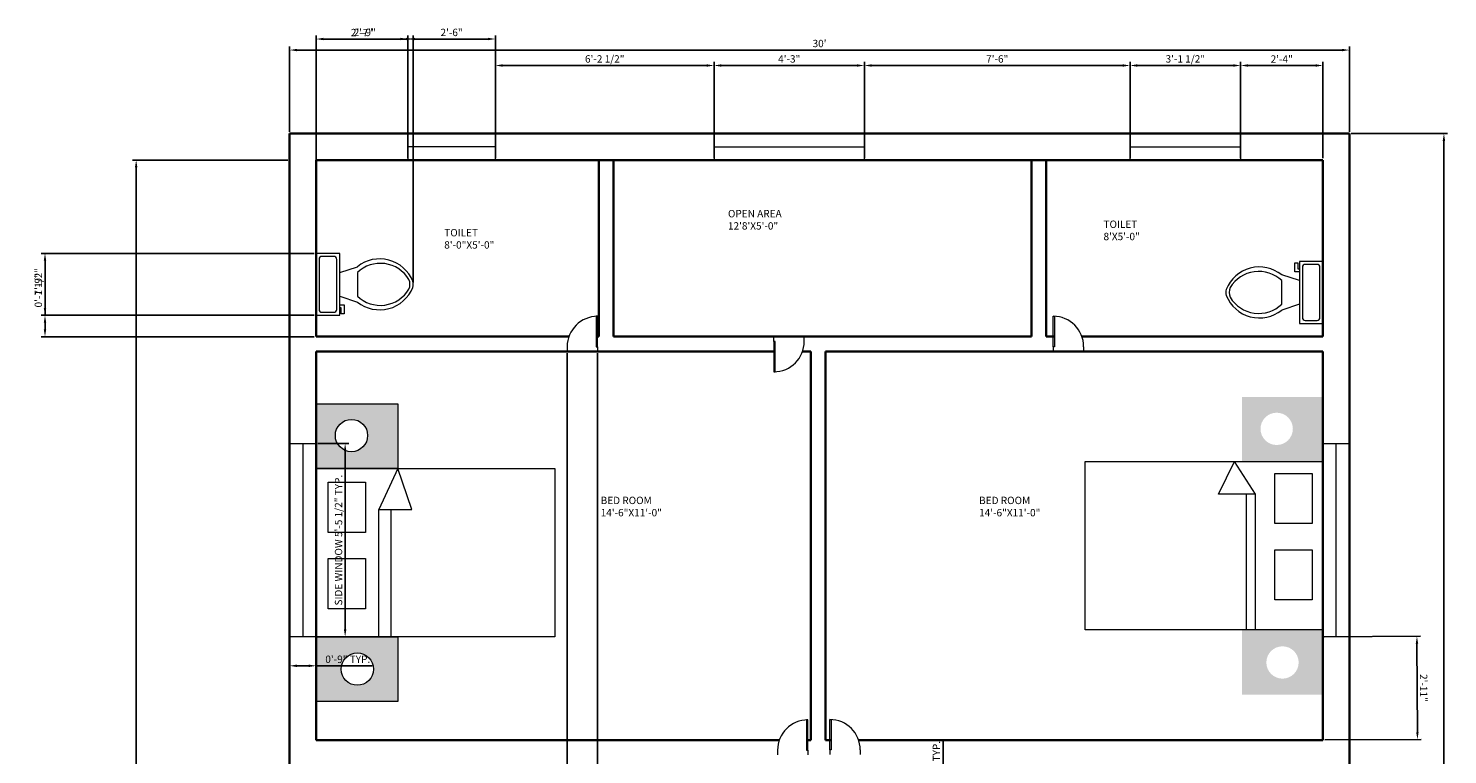
# Model space of a CAD drawing. Units: inches. Extents: x 311 to 793, y -3602 to -2932.
# Tile 3 of 3: x 311 to 793, y -3179 to -2932. Entities that reach past the tile are written whole.
import ezdxf

# ---------------------------------------------------------------- set-up
doc = ezdxf.new("R2010")
doc.units = ezdxf.units.IN
for name, color, linetype, lineweight in [('A-ANNO-DIMS', 2, 'Continuous', 18), ('A-AREA-IDEN', 7, 'Continuous', 18), ('A-DOOR', 3, 'Continuous', 18), ('A-FLOR-FIXT', 9, 'Continuous', 18), ('A-FURN', 8, 'Continuous', 18), ('A-FURN-PATT', 8, 'Continuous', 13), ('A-GLAZ', 4, 'Continuous', 18), ('A-WALL', 7, 'Continuous', 35)]:
    doc.layers.add(name, color=color, linetype=linetype, lineweight=lineweight)
doc.styles.get("Standard").update_dxf_attribs({"font": 'arial.ttf'})
doc.dimstyles.new('ISO-25', dxfattribs={"dimtxt": 2.5, "dimasz": 2.5, "dimexe": 1.25, "dimexo": 0.625, "dimtad": 1, "dimlunit": 3, "dimtxsty": 'Standard', "dimcen": 2.5, "dimadec": 0, "dimazin": 0, "dimtfac": 1, "dimtmove": 0, "dimatfit": 3, "dimfxl": 1, "dimarcsym": 0})

# ---------------------------------------------------------------- blocks, each defined once
blk = doc.blocks.new('*U5')
for p, q in [((0, 0), (0, -6)), ((-40, 0), (-40, -6))]:
    blk.add_line(p, q)
blk.add_lwpolyline([(0, 0), (0, 40), (-1.75, 40), (-1.75, 0)], close=True)
blk.add_arc((0, 0), 40, 90, 180)
blk = doc.blocks.new('*U4')
for p, q in [((0, 0), (0, 6)), ((40, 0), (40, 6))]:
    blk.add_line(p, q)
blk.add_lwpolyline([(0, 0), (0, -40), (1.75, -40), (1.75, 0)], close=True)
blk.add_arc((0, 0), 40, 270, 0)
blk = doc.blocks.new('*U2')
for p, q in [((0, 0), (0, -6)), ((40, 0), (40, -6))]:
    blk.add_line(p, q)
blk.add_lwpolyline([(0, 0), (0, 40), (1.75, 40), (1.75, 0)], close=True)
blk.add_arc((0, 0), 40, 0, 90)
blk = doc.blocks.new('*U8')
for p, q in [((9.5, -6), (9.5, -2)), ((-10, -8.5), (-8, -8.5)), ((-10, -9.5), (-10, -8.5)), ((-7, -9.5), (-10, -9.5)), ((-8, -8.5), (-8, -8)), ((-7, -8), (-7, -9.5)), ((-4, -8), (-6, -14)), ((4, -8), (6, -14)), ((4, -14), (-4, -14))]:
    blk.add_line(p, q)
blk.add_lwpolyline([(10.5, -8), (10.5, 0), (-10.5, 0), (-10.5, -8)], close=True)
for points in [[(-9.5, -2), (-9.5, -6)], [(8.5, -1), (-8.5, -1)], [(-8.5, -7), (8.5, -7)]]:
    blk.add_lwpolyline(points)
for centre, radius, start, end in [((-8.62, -1.88), 0.884, 81.8699, 188.1301), ((8.62, -1.88), 0.884, 351.8699, 98.1301), ((-8.62, -6.12), 0.884, 171.8699, 278.1301), ((8.62, -6.12), 0.884, 261.8699, 8.1301), ((3.52, -21.58), 12.17, 141.4691, 247.9714), ((4.2, -21.82), 11.33, 136.3677, 238.9468), ((-3.52, -21.58), 12.17, 292.0284, 38.5307), ((-4.2, -21.82), 11.33, 301.053, 43.6321), ((0, -27.88), 4, 245.7318, 294.2682), ((0, -29), 4, 254.8605, 285.1395)]:
    blk.add_arc(centre, radius, start, end)
blk = doc.blocks.new('*D11')
at = {"layer": 'A-ANNO-DIMS', "color": 0, "lineweight": -2, "transparency": 16777216}
for p, q in [((399.79, -2967), (399.79, -2938.03)), ((402.29, -2939.28), (757.29, -2939.28)), ((759.79, -2967), (759.79, -2938.03))]:
    blk.add_line(p, q, dxfattribs=at)
at = {"layer": 'A-ANNO-DIMS', "color": 0, "transparency": 16777216}
for points in [[(402.29, -2938.86), (402.29, -2939.7), (399.79, -2939.28)], [(757.29, -2938.86), (757.29, -2939.7), (759.79, -2939.28)]]:
    blk.add_solid(points, dxfattribs=at)
at = {"layer": 'Defpoints', "color": 0, "transparency": 16777216}
for p in [(759.79, -2939.28), (399.79, -2967.63), (759.79, -2967.63)]:
    blk.add_point(p, dxfattribs=at)
at = {"layer": 'A-ANNO-DIMS', "color": 0, "transparency": 16777216, "insert": (579.79, -2937.38), "char_height": 2.5, "attachment_point": 5}
blk.add_mtext("30'", dxfattribs=at)
blk = doc.blocks.new('*D12')
at = {"layer": 'A-ANNO-DIMS', "color": 0, "lineweight": -2, "transparency": 16777216}
for p, q in [((399.17, -2976.63), (346.4, -2976.63)), ((347.65, -2979.13), (347.65, -3565.13)), ((399.17, -3567.63), (346.4, -3567.63))]:
    blk.add_line(p, q, dxfattribs=at)
at = {"layer": 'A-ANNO-DIMS', "color": 0, "transparency": 16777216}
for points in [[(347.23, -2979.13), (348.07, -2979.13), (347.65, -2976.63)], [(347.23, -3565.13), (348.07, -3565.13), (347.65, -3567.63)]]:
    blk.add_solid(points, dxfattribs=at)
at = {"layer": 'Defpoints', "color": 0, "transparency": 16777216}
for p in [(399.79, -2976.63), (347.65, -3567.63), (399.79, -3567.63)]:
    blk.add_point(p, dxfattribs=at)
at = {"layer": 'A-ANNO-DIMS', "color": 0, "transparency": 16777216, "insert": (345.75, -3272.13), "char_height": 2.5, "attachment_point": 5, "rotation": 90}
blk.add_mtext('49\'-3"', dxfattribs=at)
blk = doc.blocks.new('WINDOW-SIDE-66')
for p, q in [((0, 65.66), (9, 65.66)), ((0, 0), (0, 65.66)), ((0, 65.66), (4.5, 65.66)), ((4.5, 65.66), (4.5, 0)), ((9, 65.66), (9, 0)), ((9, 0), (0, 0))]:
    blk.add_line(p, q)
blk = doc.blocks.new('BED-DOUBLE-WITH-NIGHTSTANDS')
h = blk.add_hatch(color=256)
h.dxf.hatch_style = 1
h.set_gradient(color1=(0, 0, 255), color2=(255, 255, 0), tint=1, name='INVSPHERICAL')
h.paths.add_polyline_path([(80.82, 21.98), (53.33, 21.98), (53.33, 0), (80.82, 0)])
h.paths.add_polyline_path([(72.57, 10.99, -1), (61.59, 10.99, -1)], flags=16)
h.paths.add_polyline_path([(80.82, 101.13), (53.33, 101.13), (53.33, 79.18), (80.82, 79.18)])
h.paths.add_polyline_path([(70.59, 90.34, -1), (59.61, 90.34, -1)], flags=16)
for p, q in [((45.33, 68.14), (50.79, 79.26)), ((57.92, 68.14), (50.79, 79.26)), ((54.79, 68.14), (45.33, 68.14)), ((57.92, 68.14), (54.79, 68.14)), ((54.79, 68.14), (54.79, 22.05)), ((57.92, 22.05), (57.92, 68.14))]:
    blk.add_line(p, q)
for points in [[(0, 79.26), (80.82, 79.26), (80.82, 22.05), (0, 22.05)], [(64.46, 75.22), (77.12, 75.22), (77.12, 58.15), (64.46, 58.15)], [(64.46, 49.29), (77.12, 49.29), (77.12, 32.22), (64.46, 32.22)]]:
    blk.add_lwpolyline(points, close=True)
blk = doc.blocks.new('*D17')
at = {"layer": 'A-ANNO-DIMS', "color": 0, "lineweight": -2, "transparency": 16777216}
for p, q in [((621.74, -3198.05), (621.74, -3173.47)), ((624.11, -3198.05), (620.49, -3198.05)), ((621.74, -3214.16), (621.74, -3200.55)), ((624.11, -3216.66), (620.49, -3216.66))]:
    blk.add_line(p, q, dxfattribs=at)
at = {"layer": 'A-ANNO-DIMS', "color": 0, "transparency": 16777216}
for points in [[(621.32, -3200.55), (622.15, -3200.55), (621.74, -3198.05)], [(621.32, -3214.16), (622.15, -3214.16), (621.74, -3216.66)]]:
    blk.add_solid(points, dxfattribs=at)
at = {"layer": 'Defpoints', "color": 0, "transparency": 16777216}
for p in [(621.74, -3198.05), (624.73, -3198.05), (624.73, -3216.66)]:
    blk.add_point(p, dxfattribs=at)
at = {"layer": 'A-ANNO-DIMS', "color": 0, "transparency": 16777216, "insert": (619.82, -3184.51), "char_height": 2.5, "attachment_point": 5, "rotation": 90}
blk.add_mtext('1\'-6 1/2" TYP.', dxfattribs=at)
blk = doc.blocks.new('*D18')
at = {"layer": 'A-ANNO-DIMS', "color": 0, "lineweight": -2, "transparency": 16777216}
for p, q in [((409.42, -3072.92), (419.89, -3072.92)), ((418.64, -3136.07), (418.64, -3075.42)), ((409.42, -3138.57), (419.89, -3138.57))]:
    blk.add_line(p, q, dxfattribs=at)
at = {"layer": 'A-ANNO-DIMS', "color": 0, "transparency": 16777216}
for points in [[(418.22, -3075.42), (419.06, -3075.42), (418.64, -3072.92)], [(418.22, -3136.07), (419.06, -3136.07), (418.64, -3138.57)]]:
    blk.add_solid(points, dxfattribs=at)
at = {"layer": 'Defpoints', "color": 0, "transparency": 16777216}
for p in [(408.79, -3072.92), (418.64, -3072.92), (408.79, -3138.57)]:
    blk.add_point(p, dxfattribs=at)
at = {"layer": 'A-ANNO-DIMS', "color": 0, "transparency": 16777216, "insert": (416.72, -3105.74), "char_height": 2.5, "attachment_point": 5, "rotation": 90}
blk.add_mtext('SIDE WINDOW 5\'-5 1/2" TYP.', dxfattribs=at)
blk = doc.blocks.new('*D19')
at = {"layer": 'A-ANNO-DIMS', "color": 0, "lineweight": -2, "transparency": 16777216}
for p, q in [((399.79, -3139.2), (399.79, -3149.67)), ((408.79, -3139.2), (408.79, -3149.67)), ((402.29, -3148.42), (406.29, -3148.42)), ((408.79, -3148.42), (427.78, -3148.42))]:
    blk.add_line(p, q, dxfattribs=at)
at = {"layer": 'A-ANNO-DIMS', "color": 0, "transparency": 16777216}
for points in [[(402.29, -3148), (402.29, -3148.84), (399.79, -3148.42)], [(406.29, -3148), (406.29, -3148.84), (408.79, -3148.42)]]:
    blk.add_solid(points, dxfattribs=at)
at = {"layer": 'Defpoints', "color": 0, "transparency": 16777216}
for p in [(399.79, -3138.57), (408.79, -3138.57), (408.79, -3148.42)]:
    blk.add_point(p, dxfattribs=at)
at = {"layer": 'A-ANNO-DIMS', "color": 0, "transparency": 16777216, "insert": (419.54, -3146.52), "char_height": 2.5, "attachment_point": 5}
blk.add_mtext('0\'-9" TYP.', dxfattribs=at)
blk = doc.blocks.new('*D24')
at = {"layer": 'A-ANNO-DIMS', "color": 0, "lineweight": -2, "transparency": 16777216}
for p, q in [((760.42, -2967.63), (793.14, -2967.63)), ((791.89, -2970.13), (791.89, -3565.13)), ((760.42, -3567.63), (793.14, -3567.63))]:
    blk.add_line(p, q, dxfattribs=at)
at = {"layer": 'A-ANNO-DIMS', "color": 0, "transparency": 16777216}
for points in [[(791.47, -2970.13), (792.31, -2970.13), (791.89, -2967.63)], [(791.47, -3565.13), (792.31, -3565.13), (791.89, -3567.63)]]:
    blk.add_solid(points, dxfattribs=at)
at = {"layer": 'Defpoints', "color": 0, "transparency": 16777216}
for p in [(759.79, -2967.63), (759.79, -3567.63), (791.89, -3567.63)]:
    blk.add_point(p, dxfattribs=at)
at = {"layer": 'A-ANNO-DIMS', "color": 0, "transparency": 16777216, "insert": (789.99, -3267.63), "char_height": 2.5, "attachment_point": 5, "rotation": 90}
blk.add_mtext('50\'-0"', dxfattribs=at)
blk = doc.blocks.new('*D34')
at = {"layer": 'A-ANNO-DIMS', "color": 0, "lineweight": -2, "transparency": 16777216}
for p, q in [((408.79, -2976), (408.79, -2934.28)), ((411.29, -2935.53), (437.41, -2935.53)), ((439.91, -2976), (439.91, -2934.28))]:
    blk.add_line(p, q, dxfattribs=at)
at = {"layer": 'A-ANNO-DIMS', "color": 0, "transparency": 16777216}
for points in [[(411.29, -2935.11), (411.29, -2935.94), (408.79, -2935.53)], [(437.41, -2935.11), (437.41, -2935.94), (439.91, -2935.53)]]:
    blk.add_solid(points, dxfattribs=at)
at = {"layer": 'Defpoints', "color": 0, "transparency": 16777216}
for p in [(439.91, -2935.53), (408.79, -2976.63), (439.91, -2976.63)]:
    blk.add_point(p, dxfattribs=at)
at = {"layer": 'A-ANNO-DIMS', "color": 0, "transparency": 16777216, "insert": (424.35, -2933.65), "char_height": 2.5, "attachment_point": 5}
blk.add_mtext('2\'-7"', dxfattribs=at)
blk = doc.blocks.new('*D35')
at = {"layer": 'A-ANNO-DIMS', "color": 0, "lineweight": -2, "transparency": 16777216}
for p, q in [((439.91, -2976), (439.91, -2934.28)), ((442.41, -2935.53), (467.18, -2935.53)), ((469.68, -2976), (469.68, -2934.28))]:
    blk.add_line(p, q, dxfattribs=at)
at = {"layer": 'A-ANNO-DIMS', "color": 0, "transparency": 16777216}
for points in [[(442.41, -2935.11), (442.41, -2935.94), (439.91, -2935.53)], [(467.18, -2935.11), (467.18, -2935.94), (469.68, -2935.53)]]:
    blk.add_solid(points, dxfattribs=at)
at = {"layer": 'Defpoints', "color": 0, "transparency": 16777216}
for p in [(469.68, -2935.53), (439.91, -2976.63), (469.68, -2976.63)]:
    blk.add_point(p, dxfattribs=at)
at = {"layer": 'A-ANNO-DIMS', "color": 0, "transparency": 16777216, "insert": (454.8, -2933.62), "char_height": 2.5, "attachment_point": 5}
blk.add_mtext('2\'-6"', dxfattribs=at)
blk = doc.blocks.new('*D36')
at = {"layer": 'A-ANNO-DIMS', "color": 0, "lineweight": -2, "transparency": 16777216}
for p, q in [((469.68, -2976), (469.68, -2943.28)), ((472.18, -2944.53), (541.47, -2944.53)), ((543.97, -2976), (543.97, -2943.28))]:
    blk.add_line(p, q, dxfattribs=at)
at = {"layer": 'A-ANNO-DIMS', "color": 0, "transparency": 16777216}
for points in [[(472.18, -2944.11), (472.18, -2944.94), (469.68, -2944.53)], [(541.47, -2944.11), (541.47, -2944.94), (543.97, -2944.53)]]:
    blk.add_solid(points, dxfattribs=at)
at = {"layer": 'Defpoints', "color": 0, "transparency": 16777216}
for p in [(543.97, -2944.53), (469.68, -2976.63), (543.97, -2976.63)]:
    blk.add_point(p, dxfattribs=at)
at = {"layer": 'A-ANNO-DIMS', "color": 0, "transparency": 16777216, "insert": (506.83, -2942.61), "char_height": 2.5, "attachment_point": 5}
blk.add_mtext('6\'-2 1/2"', dxfattribs=at)
blk = doc.blocks.new('*D37')
at = {"layer": 'A-ANNO-DIMS', "color": 0, "lineweight": -2, "transparency": 16777216}
for p, q in [((543.97, -2976), (543.97, -2943.28)), ((546.47, -2944.53), (592.53, -2944.53)), ((595.03, -2976), (595.03, -2943.28))]:
    blk.add_line(p, q, dxfattribs=at)
at = {"layer": 'A-ANNO-DIMS', "color": 0, "transparency": 16777216}
for points in [[(546.47, -2944.11), (546.47, -2944.94), (543.97, -2944.53)], [(592.53, -2944.11), (592.53, -2944.94), (595.03, -2944.53)]]:
    blk.add_solid(points, dxfattribs=at)
at = {"layer": 'Defpoints', "color": 0, "transparency": 16777216}
for p in [(595.03, -2944.53), (543.97, -2976.63), (595.03, -2976.63)]:
    blk.add_point(p, dxfattribs=at)
at = {"layer": 'A-ANNO-DIMS', "color": 0, "transparency": 16777216, "insert": (569.5, -2942.62), "char_height": 2.5, "attachment_point": 5}
blk.add_mtext('4\'-3"', dxfattribs=at)
blk = doc.blocks.new('*D38')
at = {"layer": 'A-ANNO-DIMS', "color": 0, "lineweight": -2, "transparency": 16777216}
for p, q in [((595.03, -2976), (595.03, -2943.28)), ((597.53, -2944.53), (682.77, -2944.53)), ((685.27, -2976), (685.27, -2943.28))]:
    blk.add_line(p, q, dxfattribs=at)
at = {"layer": 'A-ANNO-DIMS', "color": 0, "transparency": 16777216}
for points in [[(597.53, -2944.11), (597.53, -2944.94), (595.03, -2944.53)], [(682.77, -2944.11), (682.77, -2944.94), (685.27, -2944.53)]]:
    blk.add_solid(points, dxfattribs=at)
at = {"layer": 'Defpoints', "color": 0, "transparency": 16777216}
for p in [(685.27, -2944.53), (595.03, -2976.63), (685.27, -2976.63)]:
    blk.add_point(p, dxfattribs=at)
at = {"layer": 'A-ANNO-DIMS', "color": 0, "transparency": 16777216, "insert": (640.15, -2942.62), "char_height": 2.5, "attachment_point": 5}
blk.add_mtext('7\'-6"', dxfattribs=at)
blk = doc.blocks.new('*D39')
at = {"layer": 'A-ANNO-DIMS', "color": 0, "lineweight": -2, "transparency": 16777216}
for p, q in [((685.27, -2976), (685.27, -2943.28)), ((687.77, -2944.53), (720.31, -2944.53)), ((722.81, -2976), (722.81, -2943.28))]:
    blk.add_line(p, q, dxfattribs=at)
at = {"layer": 'A-ANNO-DIMS', "color": 0, "transparency": 16777216}
for points in [[(687.77, -2944.11), (687.77, -2944.94), (685.27, -2944.53)], [(720.31, -2944.11), (720.31, -2944.94), (722.81, -2944.53)]]:
    blk.add_solid(points, dxfattribs=at)
at = {"layer": 'Defpoints', "color": 0, "transparency": 16777216}
for p in [(722.81, -2944.53), (685.27, -2976.63), (722.81, -2976.63)]:
    blk.add_point(p, dxfattribs=at)
at = {"layer": 'A-ANNO-DIMS', "color": 0, "transparency": 16777216, "insert": (704.04, -2942.61), "char_height": 2.5, "attachment_point": 5}
blk.add_mtext('3\'-1 1/2"', dxfattribs=at)
blk = doc.blocks.new('*D40')
at = {"layer": 'A-ANNO-DIMS', "color": 0, "lineweight": -2, "transparency": 16777216}
for p, q in [((722.81, -2976), (722.81, -2943.28)), ((725.31, -2944.53), (748.29, -2944.53)), ((750.79, -2976), (750.79, -2943.28))]:
    blk.add_line(p, q, dxfattribs=at)
at = {"layer": 'A-ANNO-DIMS', "color": 0, "transparency": 16777216}
for points in [[(725.31, -2944.11), (725.31, -2944.94), (722.81, -2944.53)], [(748.29, -2944.11), (748.29, -2944.94), (750.79, -2944.53)]]:
    blk.add_solid(points, dxfattribs=at)
at = {"layer": 'Defpoints', "color": 0, "transparency": 16777216}
for p in [(750.79, -2944.53), (722.81, -2976.63), (750.79, -2976.63)]:
    blk.add_point(p, dxfattribs=at)
at = {"layer": 'A-ANNO-DIMS', "color": 0, "transparency": 16777216, "insert": (736.8, -2942.65), "char_height": 2.5, "attachment_point": 5}
blk.add_mtext('2\'-4"', dxfattribs=at)
blk = doc.blocks.new('*D42')
at = {"layer": 'A-ANNO-DIMS', "color": 0, "lineweight": -2, "transparency": 16777216}
for p, q in [((751.24, -3138.57), (783.97, -3138.41)), ((782.73, -3140.92), (782.88, -3170.97)), ((751.42, -3173.62), (784.14, -3173.46))]:
    blk.add_line(p, q, dxfattribs=at)
at = {"layer": 'A-ANNO-DIMS', "color": 0, "transparency": 16777216}
for points in [[(783.15, -3140.91), (782.31, -3140.92), (782.72, -3138.42)], [(783.3, -3170.97), (782.46, -3170.97), (782.89, -3173.47)]]:
    blk.add_solid(points, dxfattribs=at)
at = {"layer": 'Defpoints', "color": 0, "transparency": 16777216}
for p in [(750.62, -3138.57), (750.79, -3173.63), (782.89, -3173.47)]:
    blk.add_point(p, dxfattribs=at)
at = {"layer": 'A-ANNO-DIMS', "color": 0, "transparency": 16777216, "insert": (784.69, -3155.93), "char_height": 2.5, "attachment_point": 5, "rotation": 270.2799}
blk.add_mtext('2\'-11"', dxfattribs=at)
blk = doc.blocks.new('*D47')
at = {"layer": 'A-ANNO-DIMS', "color": 0, "lineweight": -2, "transparency": 16777216}
for p, q in [((408.79, -3007.73), (408.79, -2934.28)), ((411.29, -2935.53), (439.29, -2935.53)), ((441.79, -3018.23), (441.79, -2934.28))]:
    blk.add_line(p, q, dxfattribs=at)
at = {"layer": 'A-ANNO-DIMS', "color": 0, "transparency": 16777216}
for points in [[(411.29, -2935.11), (411.29, -2935.94), (408.79, -2935.53)], [(439.29, -2935.11), (439.29, -2935.94), (441.79, -2935.53)]]:
    blk.add_solid(points, dxfattribs=at)
at = {"layer": 'Defpoints', "color": 0, "transparency": 16777216}
for p in [(441.79, -2935.53), (408.79, -3008.36), (441.79, -3018.86)]:
    blk.add_point(p, dxfattribs=at)
at = {"layer": 'A-ANNO-DIMS', "color": 0, "transparency": 16777216, "insert": (425.29, -2933.62), "char_height": 2.5, "attachment_point": 5}
blk.add_mtext('2\'-9"', dxfattribs=at)
blk = doc.blocks.new('*D48')
at = {"layer": 'A-ANNO-DIMS', "color": 0, "lineweight": -2, "transparency": 16777216}
for p, q in [((408.17, -3008.36), (315.44, -3008.36)), ((316.69, -3026.86), (316.69, -3010.86)), ((408.17, -3029.36), (315.44, -3029.36))]:
    blk.add_line(p, q, dxfattribs=at)
at = {"layer": 'A-ANNO-DIMS', "color": 0, "transparency": 16777216}
for points in [[(316.27, -3010.86), (317.11, -3010.86), (316.69, -3008.36)], [(316.27, -3026.86), (317.11, -3026.86), (316.69, -3029.36)]]:
    blk.add_solid(points, dxfattribs=at)
at = {"layer": 'Defpoints', "color": 0, "transparency": 16777216}
for p in [(316.69, -3008.36), (408.79, -3008.36), (408.79, -3029.36)]:
    blk.add_point(p, dxfattribs=at)
at = {"layer": 'A-ANNO-DIMS', "color": 0, "transparency": 16777216, "insert": (314.79, -3018.86), "char_height": 2.5, "attachment_point": 5, "rotation": 90}
blk.add_mtext('1\'-9"', dxfattribs=at)
blk = doc.blocks.new('*D49')
at = {"layer": 'A-ANNO-DIMS', "color": 0, "lineweight": -2, "transparency": 16777216}
for p, q in [((316.69, -3029.36), (316.69, -3013.14)), ((408.17, -3029.36), (315.44, -3029.36)), ((316.69, -3034.13), (316.69, -3031.86)), ((408.17, -3036.63), (315.44, -3036.63))]:
    blk.add_line(p, q, dxfattribs=at)
at = {"layer": 'A-ANNO-DIMS', "color": 0, "transparency": 16777216}
for points in [[(316.27, -3031.86), (317.11, -3031.86), (316.69, -3029.36)], [(316.27, -3034.13), (317.11, -3034.13), (316.69, -3036.63)]]:
    blk.add_solid(points, dxfattribs=at)
at = {"layer": 'Defpoints', "color": 0, "transparency": 16777216}
for p in [(316.69, -3029.36), (408.79, -3029.36), (408.79, -3036.63)]:
    blk.add_point(p, dxfattribs=at)
at = {"layer": 'A-ANNO-DIMS', "color": 0, "transparency": 16777216, "insert": (314.77, -3020), "char_height": 2.5, "attachment_point": 5, "rotation": 90}
blk.add_mtext('0\'-7 1/2"', dxfattribs=at)
blk = doc.blocks.new('*D50')
at = {"layer": 'A-ANNO-DIMS', "color": 0, "lineweight": -2, "transparency": 16777216}
for p, q in [((494.06, -3042.22), (494.06, -3600.98)), ((504.38, -3042.22), (504.38, -3600.98)), ((496.56, -3599.73), (501.88, -3599.73)), ((504.38, -3599.73), (522.54, -3599.73))]:
    blk.add_line(p, q, dxfattribs=at)
at = {"layer": 'A-ANNO-DIMS', "color": 0, "transparency": 16777216}
for points in [[(496.56, -3599.31), (496.56, -3600.14), (494.06, -3599.73)], [(501.88, -3599.31), (501.88, -3600.14), (504.38, -3599.73)]]:
    blk.add_solid(points, dxfattribs=at)
at = {"layer": 'Defpoints', "color": 0, "transparency": 16777216}
for p in [(494.06, -3041.59), (504.38, -3041.59), (504.38, -3599.73)]:
    blk.add_point(p, dxfattribs=at)
at = {"layer": 'A-ANNO-DIMS', "color": 0, "transparency": 16777216, "insert": (514.71, -3597.81), "char_height": 2.5, "attachment_point": 5}
blk.add_mtext('0\'-10 1/2"', dxfattribs=at)

msp = doc.modelspace()

# ---------------------------------------------------------------- hatches: boundary and pattern name
at = {"layer": 'A-FURN-PATT'}
h = msp.add_hatch(color=256, dxfattribs=at)
h.dxf.hatch_style = 1
h.set_gradient(color1=(0, 0, 255), color2=(255, 255, 0), tint=1, name='INVSPHERICAL')
h.paths.add_polyline_path([(436.525, -3138.572), (409.038, -3138.572), (409.038, -3160.548), (436.525, -3160.548)])
h.paths.add_polyline_path([(428.27, -3149.56, -1), (417.293, -3149.56, -1)], flags=16)
h.paths.add_polyline_path([(436.525, -3059.421), (409.038, -3059.421), (409.038, -3081.364), (436.525, -3081.364)])
h.paths.add_polyline_path([(426.291, -3070.209, -1), (415.313, -3070.209, -1)], flags=16)

# ---------------------------------------------------------------- linework, layer by layer
at = {"layer": 'A-FURN'}
for p, q in [((436.525, -3081.397), (430.091, -3095.296)), ((441.255, -3095.296), (436.525, -3081.397)), ((430.091, -3138.572), (430.091, -3095.296)), ((430.091, -3095.296), (434.178, -3095.296)), ((430.091, -3095.296), (441.255, -3095.296)), ((434.178, -3095.296), (434.178, -3138.572))]:
    msp.add_line(p, q, dxfattribs=at)
for points in [[(409.038, -3059.421), (436.525, -3059.421), (436.525, -3081.397), (409.038, -3081.397)], [(409.038, -3081.364), (489.854, -3081.364), (489.854, -3138.572), (409.038, -3138.572)], [(412.893, -3086.08), (425.551, -3086.08), (425.551, -3103.151), (412.893, -3103.151)], [(412.893, -3112.002), (425.551, -3112.002), (425.551, -3129.072), (412.893, -3129.072)], [(409.038, -3138.572), (436.525, -3138.572), (436.525, -3160.548), (409.038, -3160.548)]]:
    msp.add_lwpolyline(points, close=True, dxfattribs=at)
for centre in [(420.802, -3070.209), (422.782, -3149.56)]:
    msp.add_circle(centre, 5.489, dxfattribs=at)
at = {"layer": 'A-GLAZ'}
for p, q in [((439.907, -2967.626), (439.907, -2976.626)), ((469.684, -2976.626), (469.684, -2967.626)), ((469.684, -2967.626), (469.684, -2972.126)), ((543.969, -2967.626), (543.969, -2976.626)), ((595.028, -2967.626), (543.969, -2967.626)), ((543.969, -2967.626), (543.969, -2972.126)), ((595.028, -2976.626), (595.028, -2967.626)), ((685.269, -2976.626), (685.269, -2967.626)), ((685.269, -2967.626), (685.269, -2972.126)), ((722.812, -2967.626), (722.812, -2976.626)), ((469.684, -2972.126), (439.907, -2972.126)), ((543.969, -2972.126), (595.028, -2972.126)), ((685.269, -2972.126), (722.812, -2972.126)), ((439.907, -2976.626), (469.684, -2976.626)), ((543.969, -2976.626), (595.028, -2976.626)), ((722.812, -2976.626), (685.269, -2976.626))]:
    msp.add_line(p, q, dxfattribs=at)
at = {"layer": 'A-WALL'}
for p, q in [((399.791, -2967.626), (759.791, -2967.626)), ((399.791, -3567.626), (399.791, -2967.626)), ((759.791, -2967.626), (759.791, -3567.626)), ((408.791, -2976.626), (750.791, -2976.626)), ((408.791, -3036.626), (408.791, -2976.626)), ((504.791, -3036.626), (504.791, -2976.626)), ((509.791, -3036.626), (509.791, -2976.626)), ((651.791, -3036.626), (651.791, -2976.626)), ((656.791, -3036.626), (656.791, -2976.626)), ((750.791, -2976.626), (750.791, -3036.626)), ((408.791, -3036.626), (494.508, -3036.626)), ((503.798, -3036.626), (504.791, -3036.626)), ((509.791, -3036.626), (651.791, -3036.626)), ((574.032, -3036.626), (651.791, -3036.626)), ((656.791, -3036.626), (659.632, -3036.626)), ((668.927, -3036.626), (750.791, -3036.626)), ((408.791, -3041.626), (564.728, -3041.626)), ((408.791, -3173.626), (408.791, -3041.626)), ((574.027, -3041.626), (576.791, -3041.626)), ((576.791, -3041.626), (576.791, -3173.626)), ((581.791, -3041.626), (581.791, -3173.626)), ((581.791, -3041.626), (750.791, -3041.626)), ((750.791, -3041.626), (750.791, -3173.626)), ((408.791, -3173.626), (565.988, -3173.626)), ((575.256, -3173.626), (576.791, -3173.626)), ((581.791, -3173.626), (583.747, -3173.626)), ((593.054, -3173.626), (750.791, -3173.626))]:
    msp.add_line(p, q, dxfattribs=at)

# ---------------------------------------------------------------- block references
at = {"layer": 'A-DOOR', "xscale": 0.2580993088148874, "yscale": 0.2580993088148874, "zscale": 0.2580993088148874}
for name, p in [('*U5', (504.381, -3040.045)), ('*U2', (659.18, -3040.028)), ('*U4', (564.276, -3038.234)), ('*U5', (575.86, -3177.104)), ('*U2', (583.295, -3176.995))]:
    msp.add_blockref(name, p, dxfattribs=at)
at = {"layer": 'A-FLOR-FIXT'}
for p, rotation in [((408.791, -3018.859), 89.99999999999994), ((750.791, -3021.606), 270)]:
    msp.add_blockref('*U8', p, dxfattribs=dict(at, rotation=rotation))
at = {"layer": 'A-FURN'}
msp.add_blockref('BED-DOUBLE-WITH-NIGHTSTANDS', (669.975, -3158.279), dxfattribs=at)
at = {"layer": 'A-GLAZ'}
for p in [(399.791, -3138.572), (750.62, -3138.572)]:
    msp.add_blockref('WINDOW-SIDE-66', p, dxfattribs=at)

# ---------------------------------------------------------------- texts
at = {"layer": 'A-AREA-IDEN', "char_height": 2.5, "attachment_point": 1}
for s, width, insert in [('OPEN AREA\\P12\'8\'X5\'-0"', 69.38499, (548.682, -2993.587)), ('TOILET\\P8\'X5\'-0"', 35.29407, (676.246, -2997.193)), ('TOILET\\P8\'-0"X5\'-0"', 32.28273, (452.302, -3000.054)), ('BED ROOM\\P14\'-6"X11\'-0"', 42.4231, (505.439, -3090.993)), ('BED ROOM\\P14\'-6"X11\'-0"', 42.4231, (633.994, -3090.993))]:
    msp.add_mtext_dynamic_manual_height_columns(s, width=width, gutter_width=12.5, heights=[0], dxfattribs=dict(at, insert=insert))

# ---------------------------------------------------------------- dimensions: what is measured, and where the dimension line sits
at = {"layer": 'A-ANNO-DIMS'}
for base, p1, p2, override, picture, middle in [((759.791, -2939.28), (399.791, -2967.626), (759.791, -2967.626), {"dimclrd": 0, "dimclre": 0, "dimclrt": 0}, '*D11', (579.791, -2937.378)), ((441.791, -2935.526), (408.791, -3008.359), (441.791, -3018.859), {"dimdec": 1, "dimlfac": 1, "dimrnd": 0, "dimzin": 1, "dimdsep": 46, "dimlunit": 4, "dimfrac": 2}, '*D47', (425.291, -2933.624)), ((439.907, -2935.526), (408.791, -2976.626), (439.907, -2976.626), {"dimdec": 1, "dimlfac": 1, "dimrnd": 0, "dimzin": 1, "dimdsep": 46, "dimlunit": 4, "dimfrac": 2}, '*D34', (424.349, -2933.645)), ((469.684, -2935.526), (439.907, -2976.626), (469.684, -2976.626), {"dimdec": 1, "dimlfac": 1, "dimrnd": 0, "dimzin": 1, "dimdsep": 46, "dimlunit": 4, "dimfrac": 2}, '*D35', (454.795, -2933.624)), ((543.969, -2944.526), (469.684, -2976.626), (543.969, -2976.626), {"dimdec": 1, "dimlfac": 1, "dimrnd": 0, "dimzin": 1, "dimdsep": 46, "dimlunit": 4, "dimfrac": 2}, '*D36', (506.826, -2942.608)), ((722.812, -2944.526), (685.269, -2976.626), (722.812, -2976.626), {"dimdec": 1, "dimlfac": 1, "dimrnd": 0, "dimzin": 1, "dimdsep": 46, "dimlunit": 4, "dimfrac": 2}, '*D39', (704.041, -2942.607)), ((595.028, -2944.526), (543.969, -2976.626), (595.028, -2976.626), {"dimdec": 1, "dimlfac": 1, "dimrnd": 0, "dimzin": 1, "dimdsep": 46, "dimlunit": 4, "dimfrac": 2}, '*D37', (569.498, -2942.623)), ((685.269, -2944.526), (595.028, -2976.626), (685.269, -2976.626), {"dimdec": 1, "dimlfac": 1, "dimrnd": 0, "dimzin": 1, "dimdsep": 46, "dimlunit": 4, "dimfrac": 2}, '*D38', (640.148, -2942.624)), ((750.791, -2944.526), (722.812, -2976.626), (750.791, -2976.626), {"dimdec": 1, "dimlfac": 1, "dimrnd": 0, "dimzin": 1, "dimdsep": 46, "dimlunit": 4, "dimfrac": 2}, '*D40', (736.802, -2942.645)), ((504.381, -3599.726), (494.057, -3041.593), (504.381, -3041.593), {"dimdec": 1, "dimlfac": 1, "dimrnd": 0, "dimzin": 1, "dimdsep": 46, "dimlunit": 4, "dimfrac": 2}, '*D50', (514.712, -3597.808))]:
    dim = msp.add_linear_dim(base=base, p1=p1, p2=p2, dimstyle='ISO-25', override=override, dxfattribs=at)
    dim.commit()
    dim.dimension.update_dxf_attribs({"geometry": picture, "text_midpoint": middle})
for base, p1, p2, angle, override, picture, middle in [((791.891, -3567.626), (759.791, -2967.626), (759.791, -3567.626), 270, {"dimdec": 1, "dimlfac": 1, "dimrnd": 0, "dimzin": 1, "dimdsep": 46, "dimlunit": 4, "dimfrac": 2}, '*D24', (789.99, -3267.626)), ((347.649, -3567.626), (399.791, -2976.626), (399.791, -3567.626), 90, {"dimclrd": 0, "dimclre": 0, "dimclrt": 0}, '*D12', (345.746, -3272.126)), ((316.691, -3008.359), (408.791, -3029.359), (408.791, -3008.359), 90, {"dimdec": 1, "dimlfac": 1, "dimrnd": 0, "dimzin": 1, "dimdsep": 46, "dimlunit": 4, "dimfrac": 2}, '*D48', (314.79, -3018.859)), ((316.691, -3029.359), (408.791, -3036.626), (408.791, -3029.359), 90, {"dimdec": 1, "dimlfac": 1, "dimrnd": 0, "dimzin": 1, "dimdsep": 46, "dimlunit": 4, "dimfrac": 2}, '*D49', (314.773, -3019.999)), ((782.891, -3173.469), (750.62, -3138.572), (750.791, -3173.626), 270.27988, {"dimdec": 1, "dimlfac": 1, "dimrnd": 0, "dimzin": 1, "dimdsep": 46, "dimlunit": 4, "dimfrac": 2}, '*D42', (784.685, -3155.933))]:
    dim = msp.add_linear_dim(base=base, p1=p1, p2=p2, angle=angle, dimstyle='ISO-25', override=override, dxfattribs=at)
    dim.commit()
    dim.dimension.update_dxf_attribs({"geometry": picture, "text_midpoint": middle})
for base, p1, p2, text, picture, middle in [((418.64, -3072.915), (408.791, -3138.572), (408.791, -3072.915), 'SIDE WINDOW <> TYP.', '*D18', (416.721, -3105.744)), ((621.737, -3198.052), (624.734, -3216.663), (624.734, -3198.052), '<> TYP.', '*D17', (619.819, -3184.512))]:
    dim = msp.add_linear_dim(base=base, p1=p1, p2=p2, angle=90, text=text, dimstyle='ISO-25', override={"dimdec": 1, "dimlfac": 1, "dimrnd": 0, "dimzin": 1, "dimdsep": 46, "dimlunit": 4, "dimfrac": 2}, dxfattribs=at)
    dim.commit()
    dim.dimension.update_dxf_attribs({"geometry": picture, "text_midpoint": middle})
dim = msp.add_linear_dim(base=(408.791, -3148.421), p1=(399.791, -3138.572), p2=(408.791, -3138.572), text='<> TYP.', dimstyle='ISO-25', override={"dimdec": 1, "dimlfac": 1, "dimrnd": 0, "dimzin": 1, "dimdsep": 46, "dimlunit": 4, "dimfrac": 2}, dxfattribs=at)
dim.commit()
dim.dimension.update_dxf_attribs({"geometry": '*D19', "text_midpoint": (419.535, -3146.52)})

doc.saveas('drawing.dxf')
